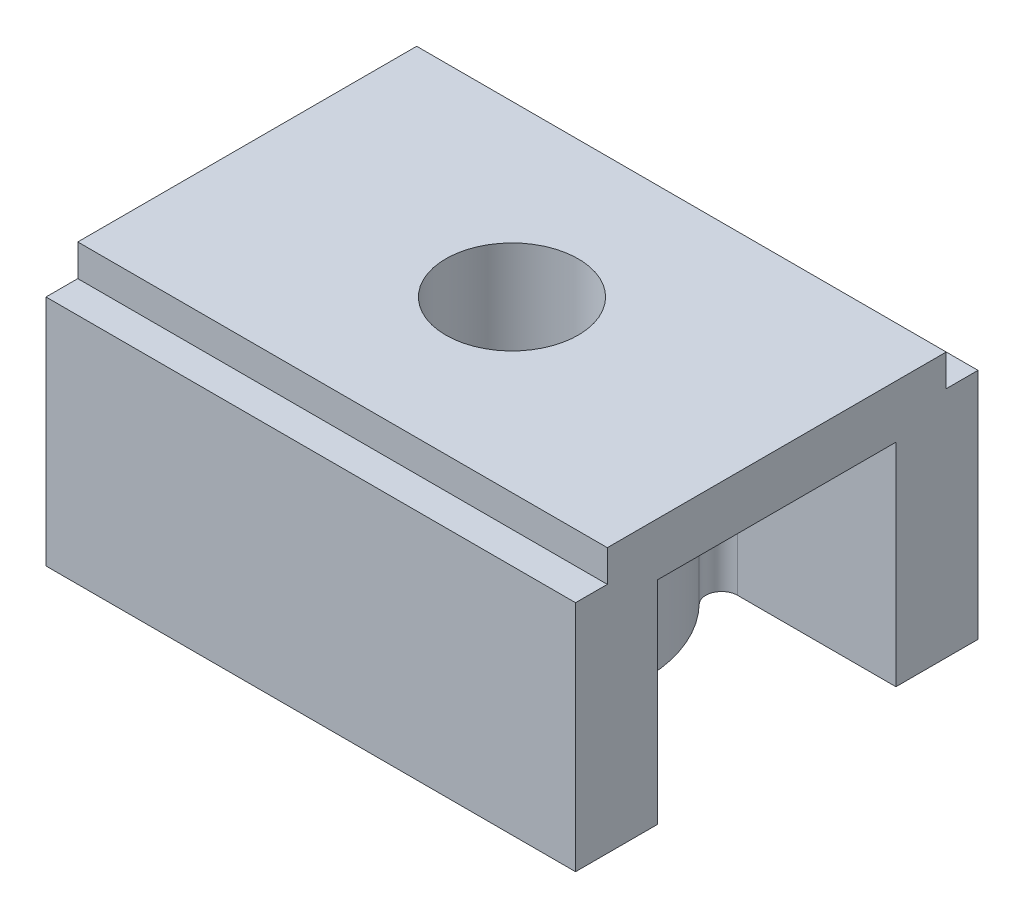
ISO-10303-21;
HEADER;
FILE_DESCRIPTION(('STEP AP214'),'2;1');
FILE_NAME('part.step','',(''),(''),'','','');
FILE_SCHEMA(('AUTOMOTIVE_DESIGN { 1 0 10303 214 1 1 1 1 }'));
ENDSEC;
DATA;
#1=APPLICATION_CONTEXT('core data for automotive mechanical design processes');
#2=APPLICATION_PROTOCOL_DEFINITION('international standard','automotive_design',2000,#1);
#3=PRODUCT_CONTEXT('',#1,'mechanical');
#4=PRODUCT('Part','Part','',(#3));
#5=PRODUCT_RELATED_PRODUCT_CATEGORY('part','',(#4));
#6=PRODUCT_DEFINITION_FORMATION('','',#4);
#7=PRODUCT_DEFINITION_CONTEXT('part definition',#1,'design');
#8=PRODUCT_DEFINITION('design','',#6,#7);
#9=PRODUCT_DEFINITION_SHAPE('','',#8);
#10=(LENGTH_UNIT() NAMED_UNIT(*) SI_UNIT(.MILLI.,.METRE.));
#11=(NAMED_UNIT(*) PLANE_ANGLE_UNIT() SI_UNIT($,.RADIAN.));
#12=(NAMED_UNIT(*) SI_UNIT($,.STERADIAN.) SOLID_ANGLE_UNIT());
#13=UNCERTAINTY_MEASURE_WITH_UNIT(LENGTH_MEASURE(1.E-05),#10,'distance_accuracy_value','');
#14=(GEOMETRIC_REPRESENTATION_CONTEXT(3) GLOBAL_UNCERTAINTY_ASSIGNED_CONTEXT((#13)) GLOBAL_UNIT_ASSIGNED_CONTEXT((#10,
#11,#12)) REPRESENTATION_CONTEXT('',''));
#15=CARTESIAN_POINT('',(0.,0.,0.));
#16=DIRECTION('',(0.,0.,1.));
#17=DIRECTION('',(1.,0.,0.));
#18=AXIS2_PLACEMENT_3D('',#15,#16,#17);
#19=CARTESIAN_POINT('',(-50.,40.,-38.));
#20=DIRECTION('',(0.,0.,-1.));
#21=DIRECTION('',(-1.,0.,0.));
#22=AXIS2_PLACEMENT_3D('',#19,#20,#21);
#23=PLANE('',#22);
#24=DIRECTION('',(0.,-1.,0.));
#25=VECTOR('',#24,1.);
#26=CARTESIAN_POINT('',(-50.,40.,-38.));
#27=LINE('',#26,#25);
#28=CARTESIAN_POINT('',(-50.,44.,-38.));
#29=VERTEX_POINT('',#28);
#30=CARTESIAN_POINT('',(-50.,0.,-38.));
#31=VERTEX_POINT('',#30);
#32=EDGE_CURVE('E195',#29,#31,#27,.T.);
#33=ORIENTED_EDGE('',*,*,#32,.F.);
#34=DIRECTION('',(-1.,0.,0.));
#35=VECTOR('',#34,1.);
#36=CARTESIAN_POINT('',(50.,44.,-38.));
#37=LINE('',#36,#35);
#38=CARTESIAN_POINT('',(50.,44.,-38.));
#39=VERTEX_POINT('',#38);
#40=EDGE_CURVE('E177',#39,#29,#37,.T.);
#41=ORIENTED_EDGE('',*,*,#40,.F.);
#42=DIRECTION('',(0.,-1.,0.));
#43=VECTOR('',#42,1.);
#44=CARTESIAN_POINT('',(50.,40.,-38.));
#45=LINE('',#44,#43);
#46=CARTESIAN_POINT('',(50.,0.,-38.));
#47=VERTEX_POINT('',#46);
#48=EDGE_CURVE('E188',#39,#47,#45,.T.);
#49=ORIENTED_EDGE('',*,*,#48,.T.);
#50=DIRECTION('',(1.,0.,0.));
#51=VECTOR('',#50,1.);
#52=CARTESIAN_POINT('',(-50.,0.,-38.));
#53=LINE('',#52,#51);
#54=EDGE_CURVE('E253',#31,#47,#53,.T.);
#55=ORIENTED_EDGE('',*,*,#54,.F.);
#56=EDGE_LOOP('',(#33,#41,#49,#55));
#57=FACE_BOUND('',#56,.T.);
#58=ADVANCED_FACE('F39',(#57),#23,.T.);
#59=CARTESIAN_POINT('',(-50.,40.,38.));
#60=DIRECTION('',(0.,0.,-1.));
#61=DIRECTION('',(-1.,0.,0.));
#62=AXIS2_PLACEMENT_3D('',#59,#60,#61);
#63=PLANE('',#62);
#64=DIRECTION('',(0.,-1.,0.));
#65=VECTOR('',#64,1.);
#66=CARTESIAN_POINT('',(50.,40.,38.));
#67=LINE('',#66,#65);
#68=CARTESIAN_POINT('',(50.,44.,38.));
#69=VERTEX_POINT('',#68);
#70=CARTESIAN_POINT('',(50.,0.,38.));
#71=VERTEX_POINT('',#70);
#72=EDGE_CURVE('E50',#69,#71,#67,.T.);
#73=ORIENTED_EDGE('',*,*,#72,.F.);
#74=DIRECTION('',(1.,0.,0.));
#75=VECTOR('',#74,1.);
#76=CARTESIAN_POINT('',(-50.,44.,38.));
#77=LINE('',#76,#75);
#78=CARTESIAN_POINT('',(-50.,44.,38.));
#79=VERTEX_POINT('',#78);
#80=EDGE_CURVE('E539',#79,#69,#77,.T.);
#81=ORIENTED_EDGE('',*,*,#80,.F.);
#82=DIRECTION('',(0.,-1.,0.));
#83=VECTOR('',#82,1.);
#84=CARTESIAN_POINT('',(-50.,40.,38.));
#85=LINE('',#84,#83);
#86=CARTESIAN_POINT('',(-50.,0.,38.));
#87=VERTEX_POINT('',#86);
#88=EDGE_CURVE('E11',#79,#87,#85,.T.);
#89=ORIENTED_EDGE('',*,*,#88,.T.);
#90=DIRECTION('',(1.,0.,0.));
#91=VECTOR('',#90,1.);
#92=CARTESIAN_POINT('',(-50.,0.,38.));
#93=LINE('',#92,#91);
#94=EDGE_CURVE('E226',#87,#71,#93,.T.);
#95=ORIENTED_EDGE('',*,*,#94,.T.);
#96=EDGE_LOOP('',(#73,#81,#89,#95));
#97=FACE_BOUND('',#96,.T.);
#98=ADVANCED_FACE('F41',(#97),#63,.F.);
#99=CARTESIAN_POINT('',(20.0935312974101,40.,22.5));
#100=DIRECTION('',(0.,0.,-1.));
#101=DIRECTION('',(-1.,0.,0.));
#102=AXIS2_PLACEMENT_3D('',#99,#100,#101);
#103=PLANE('',#102);
#104=DIRECTION('',(1.,0.,0.));
#105=VECTOR('',#104,1.);
#106=CARTESIAN_POINT('',(20.0935312974101,0.,22.5));
#107=LINE('',#106,#105);
#108=CARTESIAN_POINT('',(20.0935312974101,0.,22.5));
#109=VERTEX_POINT('',#108);
#110=CARTESIAN_POINT('',(50.,0.,22.5));
#111=VERTEX_POINT('',#110);
#112=EDGE_CURVE('E238',#109,#111,#107,.T.);
#113=ORIENTED_EDGE('',*,*,#112,.F.);
#114=DIRECTION('',(0.,-1.,0.));
#115=VECTOR('',#114,1.);
#116=CARTESIAN_POINT('',(20.0935312974101,40.,22.5));
#117=LINE('',#116,#115);
#118=CARTESIAN_POINT('',(20.0935312974101,40.,22.5));
#119=VERTEX_POINT('',#118);
#120=EDGE_CURVE('E215',#119,#109,#117,.T.);
#121=ORIENTED_EDGE('',*,*,#120,.F.);
#122=DIRECTION('',(1.,0.,0.));
#123=VECTOR('',#122,1.);
#124=CARTESIAN_POINT('',(20.0935312974101,40.,22.5));
#125=LINE('',#124,#123);
#126=CARTESIAN_POINT('',(50.,40.,22.5));
#127=VERTEX_POINT('',#126);
#128=EDGE_CURVE('E274',#119,#127,#125,.T.);
#129=ORIENTED_EDGE('',*,*,#128,.T.);
#130=DIRECTION('',(0.,-1.,0.));
#131=VECTOR('',#130,1.);
#132=CARTESIAN_POINT('',(50.,40.,22.5));
#133=LINE('',#132,#131);
#134=EDGE_CURVE('E211',#127,#111,#133,.T.);
#135=ORIENTED_EDGE('',*,*,#134,.T.);
#136=EDGE_LOOP('',(#113,#121,#129,#135));
#137=FACE_BOUND('',#136,.T.);
#138=ADVANCED_FACE('F361',(#137),#103,.T.);
#139=CARTESIAN_POINT('',(20.0935312974101,40.,19.5));
#140=DIRECTION('',(0.,-1.,0.));
#141=DIRECTION('',(0.,0.,-1.));
#142=AXIS2_PLACEMENT_3D('',#139,#140,#141);
#143=CYLINDRICAL_SURFACE('',#142,3.);
#144=CARTESIAN_POINT('',(20.0935312974101,0.,19.5));
#145=DIRECTION('',(0.,1.,0.));
#146=DIRECTION('',(0.,0.,1.));
#147=AXIS2_PLACEMENT_3D('',#144,#145,#146);
#148=CIRCLE('',#147,3.);
#149=CARTESIAN_POINT('',(17.9406529441162,0.,17.4107142857143));
#150=VERTEX_POINT('',#149);
#151=EDGE_CURVE('E239',#150,#109,#148,.T.);
#152=ORIENTED_EDGE('',*,*,#151,.F.);
#153=DIRECTION('',(0.,-1.,0.));
#154=VECTOR('',#153,1.);
#155=CARTESIAN_POINT('',(17.9406529441162,40.,17.4107142857143));
#156=LINE('',#155,#154);
#157=CARTESIAN_POINT('',(17.9406529441162,40.,17.4107142857143));
#158=VERTEX_POINT('',#157);
#159=EDGE_CURVE('E208',#158,#150,#156,.T.);
#160=ORIENTED_EDGE('',*,*,#159,.F.);
#161=CARTESIAN_POINT('',(20.0935312974101,40.,19.5));
#162=DIRECTION('',(0.,1.,0.));
#163=DIRECTION('',(0.,0.,1.));
#164=AXIS2_PLACEMENT_3D('',#161,#162,#163);
#165=CIRCLE('',#164,3.);
#166=EDGE_CURVE('E332',#158,#119,#165,.T.);
#167=ORIENTED_EDGE('',*,*,#166,.T.);
#168=ORIENTED_EDGE('',*,*,#120,.T.);
#169=EDGE_LOOP('',(#152,#160,#167,#168));
#170=FACE_BOUND('',#169,.T.);
#171=ADVANCED_FACE('F359',(#170),#143,.F.);
#172=CARTESIAN_POINT('',(0.,40.,0.));
#173=DIRECTION('',(0.,-1.,0.));
#174=DIRECTION('',(0.,0.,-1.));
#175=AXIS2_PLACEMENT_3D('',#172,#173,#174);
#176=CYLINDRICAL_SURFACE('',#175,25.);
#177=CARTESIAN_POINT('',(0.,0.,0.));
#178=DIRECTION('',(0.,1.,0.));
#179=DIRECTION('',(0.,0.,1.));
#180=AXIS2_PLACEMENT_3D('',#177,#178,#179);
#181=CIRCLE('',#180,25.);
#182=CARTESIAN_POINT('',(17.9406529441162,0.,-17.4107142857143));
#183=VERTEX_POINT('',#182);
#184=EDGE_CURVE('E244',#150,#183,#181,.T.);
#185=ORIENTED_EDGE('',*,*,#184,.T.);
#186=DIRECTION('',(0.,-1.,0.));
#187=VECTOR('',#186,1.);
#188=CARTESIAN_POINT('',(17.9406529441162,40.,-17.4107142857143));
#189=LINE('',#188,#187);
#190=CARTESIAN_POINT('',(17.9406529441162,40.,-17.4107142857143));
#191=VERTEX_POINT('',#190);
#192=EDGE_CURVE('E206',#191,#183,#189,.T.);
#193=ORIENTED_EDGE('',*,*,#192,.F.);
#194=CARTESIAN_POINT('',(0.,40.,0.));
#195=DIRECTION('',(0.,1.,0.));
#196=DIRECTION('',(0.,0.,1.));
#197=AXIS2_PLACEMENT_3D('',#194,#195,#196);
#198=CIRCLE('',#197,25.);
#199=EDGE_CURVE('E340',#158,#191,#198,.T.);
#200=ORIENTED_EDGE('',*,*,#199,.F.);
#201=ORIENTED_EDGE('',*,*,#159,.T.);
#202=EDGE_LOOP('',(#185,#193,#200,#201));
#203=FACE_BOUND('',#202,.T.);
#204=ADVANCED_FACE('F358',(#203),#176,.T.);
#205=CARTESIAN_POINT('',(20.0935312974101,40.,-19.5));
#206=DIRECTION('',(0.,-1.,0.));
#207=DIRECTION('',(0.,0.,-1.));
#208=AXIS2_PLACEMENT_3D('',#205,#206,#207);
#209=CYLINDRICAL_SURFACE('',#208,3.);
#210=CARTESIAN_POINT('',(20.0935312974101,0.,-19.5));
#211=DIRECTION('',(0.,1.,0.));
#212=DIRECTION('',(0.,0.,1.));
#213=AXIS2_PLACEMENT_3D('',#210,#211,#212);
#214=CIRCLE('',#213,3.);
#215=CARTESIAN_POINT('',(20.0935312974101,0.,-22.5));
#216=VERTEX_POINT('',#215);
#217=EDGE_CURVE('E247',#216,#183,#214,.T.);
#218=ORIENTED_EDGE('',*,*,#217,.F.);
#219=DIRECTION('',(0.,-1.,0.));
#220=VECTOR('',#219,1.);
#221=CARTESIAN_POINT('',(20.0935312974101,40.,-22.5));
#222=LINE('',#221,#220);
#223=CARTESIAN_POINT('',(20.0935312974101,40.,-22.5));
#224=VERTEX_POINT('',#223);
#225=EDGE_CURVE('E201',#224,#216,#222,.T.);
#226=ORIENTED_EDGE('',*,*,#225,.F.);
#227=CARTESIAN_POINT('',(20.0935312974101,40.,-19.5));
#228=DIRECTION('',(0.,1.,0.));
#229=DIRECTION('',(0.,0.,1.));
#230=AXIS2_PLACEMENT_3D('',#227,#228,#229);
#231=CIRCLE('',#230,3.);
#232=EDGE_CURVE('E339',#224,#191,#231,.T.);
#233=ORIENTED_EDGE('',*,*,#232,.T.);
#234=ORIENTED_EDGE('',*,*,#192,.T.);
#235=EDGE_LOOP('',(#218,#226,#233,#234));
#236=FACE_BOUND('',#235,.T.);
#237=ADVANCED_FACE('F355',(#236),#209,.F.);
#238=CARTESIAN_POINT('',(20.0935312974101,40.,-22.5));
#239=DIRECTION('',(0.,0.,-1.));
#240=DIRECTION('',(-1.,0.,0.));
#241=AXIS2_PLACEMENT_3D('',#238,#239,#240);
#242=PLANE('',#241);
#243=DIRECTION('',(1.,0.,0.));
#244=VECTOR('',#243,1.);
#245=CARTESIAN_POINT('',(20.0935312974101,0.,-22.5));
#246=LINE('',#245,#244);
#247=CARTESIAN_POINT('',(50.,0.,-22.5));
#248=VERTEX_POINT('',#247);
#249=EDGE_CURVE('E252',#216,#248,#246,.T.);
#250=ORIENTED_EDGE('',*,*,#249,.T.);
#251=DIRECTION('',(0.,-1.,0.));
#252=VECTOR('',#251,1.);
#253=CARTESIAN_POINT('',(50.,40.,-22.5));
#254=LINE('',#253,#252);
#255=CARTESIAN_POINT('',(50.,40.,-22.5));
#256=VERTEX_POINT('',#255);
#257=EDGE_CURVE('E196',#256,#248,#254,.T.);
#258=ORIENTED_EDGE('',*,*,#257,.F.);
#259=DIRECTION('',(1.,0.,0.));
#260=VECTOR('',#259,1.);
#261=CARTESIAN_POINT('',(20.0935312974101,40.,-22.5));
#262=LINE('',#261,#260);
#263=EDGE_CURVE('E307',#224,#256,#262,.T.);
#264=ORIENTED_EDGE('',*,*,#263,.F.);
#265=ORIENTED_EDGE('',*,*,#225,.T.);
#266=EDGE_LOOP('',(#250,#258,#264,#265));
#267=FACE_BOUND('',#266,.T.);
#268=ADVANCED_FACE('F350',(#267),#242,.F.);
#269=CARTESIAN_POINT('',(50.,40.,-38.));
#270=DIRECTION('',(1.,0.,0.));
#271=DIRECTION('',(0.,0.,-1.));
#272=AXIS2_PLACEMENT_3D('',#269,#270,#271);
#273=PLANE('',#272);
#274=DIRECTION('',(0.,1.,0.));
#275=VECTOR('',#274,1.);
#276=CARTESIAN_POINT('',(50.,44.,-32.));
#277=LINE('',#276,#275);
#278=CARTESIAN_POINT('',(50.,44.,-32.));
#279=VERTEX_POINT('',#278);
#280=CARTESIAN_POINT('',(50.,50.,-32.));
#281=VERTEX_POINT('',#280);
#282=EDGE_CURVE('E532',#279,#281,#277,.T.);
#283=ORIENTED_EDGE('',*,*,#282,.T.);
#284=DIRECTION('',(0.,0.,-1.));
#285=VECTOR('',#284,1.);
#286=CARTESIAN_POINT('',(50.,50.,-38.));
#287=LINE('',#286,#285);
#288=CARTESIAN_POINT('',(50.,50.,32.));
#289=VERTEX_POINT('',#288);
#290=EDGE_CURVE('E319',#289,#281,#287,.T.);
#291=ORIENTED_EDGE('',*,*,#290,.F.);
#292=DIRECTION('',(0.,1.,0.));
#293=VECTOR('',#292,1.);
#294=CARTESIAN_POINT('',(50.,44.,32.));
#295=LINE('',#294,#293);
#296=CARTESIAN_POINT('',(50.,44.,32.));
#297=VERTEX_POINT('',#296);
#298=EDGE_CURVE('E65',#297,#289,#295,.T.);
#299=ORIENTED_EDGE('',*,*,#298,.F.);
#300=DIRECTION('',(0.,0.,-1.));
#301=VECTOR('',#300,1.);
#302=CARTESIAN_POINT('',(50.,44.,38.));
#303=LINE('',#302,#301);
#304=EDGE_CURVE('E222',#69,#297,#303,.T.);
#305=ORIENTED_EDGE('',*,*,#304,.F.);
#306=ORIENTED_EDGE('',*,*,#72,.T.);
#307=DIRECTION('',(0.,0.,1.));
#308=VECTOR('',#307,1.);
#309=CARTESIAN_POINT('',(50.,0.,22.5));
#310=LINE('',#309,#308);
#311=EDGE_CURVE('E221',#111,#71,#310,.T.);
#312=ORIENTED_EDGE('',*,*,#311,.F.);
#313=ORIENTED_EDGE('',*,*,#134,.F.);
#314=DIRECTION('',(0.,0.,-1.));
#315=VECTOR('',#314,1.);
#316=CARTESIAN_POINT('',(50.,40.,-38.));
#317=LINE('',#316,#315);
#318=EDGE_CURVE('E330',#127,#256,#317,.T.);
#319=ORIENTED_EDGE('',*,*,#318,.T.);
#320=ORIENTED_EDGE('',*,*,#257,.T.);
#321=DIRECTION('',(0.,0.,1.));
#322=VECTOR('',#321,1.);
#323=CARTESIAN_POINT('',(50.,0.,-38.));
#324=LINE('',#323,#322);
#325=EDGE_CURVE('E200',#47,#248,#324,.T.);
#326=ORIENTED_EDGE('',*,*,#325,.F.);
#327=ORIENTED_EDGE('',*,*,#48,.F.);
#328=DIRECTION('',(0.,0.,-1.));
#329=VECTOR('',#328,1.);
#330=CARTESIAN_POINT('',(50.,44.,-32.));
#331=LINE('',#330,#329);
#332=EDGE_CURVE('E176',#279,#39,#331,.T.);
#333=ORIENTED_EDGE('',*,*,#332,.F.);
#334=EDGE_LOOP('',(#283,#291,#299,#305,#306,#312,#313,#319,#320,#326,#327,#333));
#335=FACE_BOUND('',#334,.T.);
#336=ADVANCED_FACE('F193',(#335),#273,.T.);
#337=CARTESIAN_POINT('',(-50.,40.,-38.));
#338=DIRECTION('',(1.,0.,0.));
#339=DIRECTION('',(0.,0.,-1.));
#340=AXIS2_PLACEMENT_3D('',#337,#338,#339);
#341=PLANE('',#340);
#342=DIRECTION('',(0.,0.,1.));
#343=VECTOR('',#342,1.);
#344=CARTESIAN_POINT('',(-50.,50.,-38.));
#345=LINE('',#344,#343);
#346=CARTESIAN_POINT('',(-50.,50.,-32.));
#347=VERTEX_POINT('',#346);
#348=CARTESIAN_POINT('',(-50.,50.,32.));
#349=VERTEX_POINT('',#348);
#350=EDGE_CURVE('E317',#347,#349,#345,.T.);
#351=ORIENTED_EDGE('',*,*,#350,.F.);
#352=DIRECTION('',(0.,1.,0.));
#353=VECTOR('',#352,1.);
#354=CARTESIAN_POINT('',(-50.,44.,-32.));
#355=LINE('',#354,#353);
#356=CARTESIAN_POINT('',(-50.,44.,-32.));
#357=VERTEX_POINT('',#356);
#358=EDGE_CURVE('E53',#357,#347,#355,.T.);
#359=ORIENTED_EDGE('',*,*,#358,.F.);
#360=DIRECTION('',(0.,0.,1.));
#361=VECTOR('',#360,1.);
#362=CARTESIAN_POINT('',(-50.,44.,-38.));
#363=LINE('',#362,#361);
#364=EDGE_CURVE('E194',#29,#357,#363,.T.);
#365=ORIENTED_EDGE('',*,*,#364,.F.);
#366=ORIENTED_EDGE('',*,*,#32,.T.);
#367=DIRECTION('',(0.,0.,1.));
#368=VECTOR('',#367,1.);
#369=CARTESIAN_POINT('',(-50.,0.,-38.));
#370=LINE('',#369,#368);
#371=CARTESIAN_POINT('',(-50.,0.,-22.5));
#372=VERTEX_POINT('',#371);
#373=EDGE_CURVE('E260',#31,#372,#370,.T.);
#374=ORIENTED_EDGE('',*,*,#373,.T.);
#375=DIRECTION('',(0.,-1.,0.));
#376=VECTOR('',#375,1.);
#377=CARTESIAN_POINT('',(-50.,40.,-22.5));
#378=LINE('',#377,#376);
#379=CARTESIAN_POINT('',(-50.,40.,-22.5));
#380=VERTEX_POINT('',#379);
#381=EDGE_CURVE('E203',#380,#372,#378,.T.);
#382=ORIENTED_EDGE('',*,*,#381,.F.);
#383=DIRECTION('',(0.,0.,1.));
#384=VECTOR('',#383,1.);
#385=CARTESIAN_POINT('',(-50.,40.,-38.));
#386=LINE('',#385,#384);
#387=CARTESIAN_POINT('',(-50.,40.,22.5));
#388=VERTEX_POINT('',#387);
#389=EDGE_CURVE('E324',#380,#388,#386,.T.);
#390=ORIENTED_EDGE('',*,*,#389,.T.);
#391=DIRECTION('',(0.,-1.,0.));
#392=VECTOR('',#391,1.);
#393=CARTESIAN_POINT('',(-50.,40.,22.5));
#394=LINE('',#393,#392);
#395=CARTESIAN_POINT('',(-50.,0.,22.5));
#396=VERTEX_POINT('',#395);
#397=EDGE_CURVE('E273',#388,#396,#394,.T.);
#398=ORIENTED_EDGE('',*,*,#397,.T.);
#399=DIRECTION('',(0.,0.,1.));
#400=VECTOR('',#399,1.);
#401=CARTESIAN_POINT('',(-50.,0.,22.5));
#402=LINE('',#401,#400);
#403=EDGE_CURVE('E231',#396,#87,#402,.T.);
#404=ORIENTED_EDGE('',*,*,#403,.T.);
#405=ORIENTED_EDGE('',*,*,#88,.F.);
#406=DIRECTION('',(0.,0.,1.));
#407=VECTOR('',#406,1.);
#408=CARTESIAN_POINT('',(-50.,44.,32.));
#409=LINE('',#408,#407);
#410=CARTESIAN_POINT('',(-50.,44.,32.));
#411=VERTEX_POINT('',#410);
#412=EDGE_CURVE('E541',#411,#79,#409,.T.);
#413=ORIENTED_EDGE('',*,*,#412,.F.);
#414=DIRECTION('',(0.,1.,0.));
#415=VECTOR('',#414,1.);
#416=CARTESIAN_POINT('',(-50.,44.,32.));
#417=LINE('',#416,#415);
#418=EDGE_CURVE('E540',#411,#349,#417,.T.);
#419=ORIENTED_EDGE('',*,*,#418,.T.);
#420=EDGE_LOOP('',(#351,#359,#365,#366,#374,#382,#390,#398,#404,#405,#413,#419));
#421=FACE_BOUND('',#420,.T.);
#422=ADVANCED_FACE('F380',(#421),#341,.F.);
#423=CARTESIAN_POINT('',(-50.,40.,-22.5));
#424=DIRECTION('',(0.,0.,-1.));
#425=DIRECTION('',(-1.,0.,0.));
#426=AXIS2_PLACEMENT_3D('',#423,#424,#425);
#427=PLANE('',#426);
#428=DIRECTION('',(1.,0.,0.));
#429=VECTOR('',#428,1.);
#430=CARTESIAN_POINT('',(-50.,0.,-22.5));
#431=LINE('',#430,#429);
#432=CARTESIAN_POINT('',(-20.0935312974102,0.,-22.5));
#433=VERTEX_POINT('',#432);
#434=EDGE_CURVE('E256',#372,#433,#431,.T.);
#435=ORIENTED_EDGE('',*,*,#434,.T.);
#436=DIRECTION('',(0.,-1.,0.));
#437=VECTOR('',#436,1.);
#438=CARTESIAN_POINT('',(-20.0935312974102,40.,-22.5));
#439=LINE('',#438,#437);
#440=CARTESIAN_POINT('',(-20.0935312974102,40.,-22.5));
#441=VERTEX_POINT('',#440);
#442=EDGE_CURVE('E281',#441,#433,#439,.T.);
#443=ORIENTED_EDGE('',*,*,#442,.F.);
#444=DIRECTION('',(1.,0.,0.));
#445=VECTOR('',#444,1.);
#446=CARTESIAN_POINT('',(-50.,40.,-22.5));
#447=LINE('',#446,#445);
#448=EDGE_CURVE('E292',#380,#441,#447,.T.);
#449=ORIENTED_EDGE('',*,*,#448,.F.);
#450=ORIENTED_EDGE('',*,*,#381,.T.);
#451=EDGE_LOOP('',(#435,#443,#449,#450));
#452=FACE_BOUND('',#451,.T.);
#453=ADVANCED_FACE('F289',(#452),#427,.F.);
#454=CARTESIAN_POINT('',(-20.0935312974102,40.,-19.5));
#455=DIRECTION('',(0.,-1.,0.));
#456=DIRECTION('',(0.,0.,-1.));
#457=AXIS2_PLACEMENT_3D('',#454,#455,#456);
#458=CYLINDRICAL_SURFACE('',#457,3.00000000000001);
#459=CARTESIAN_POINT('',(-20.0935312974102,0.,-19.5));
#460=DIRECTION('',(0.,1.,0.));
#461=DIRECTION('',(0.,0.,1.));
#462=AXIS2_PLACEMENT_3D('',#459,#460,#461);
#463=CIRCLE('',#462,3.00000000000001);
#464=CARTESIAN_POINT('',(-17.9406529441162,0.,-17.4107142857143));
#465=VERTEX_POINT('',#464);
#466=EDGE_CURVE('E265',#465,#433,#463,.T.);
#467=ORIENTED_EDGE('',*,*,#466,.F.);
#468=DIRECTION('',(0.,-1.,0.));
#469=VECTOR('',#468,1.);
#470=CARTESIAN_POINT('',(-17.9406529441162,40.,-17.4107142857143));
#471=LINE('',#470,#469);
#472=CARTESIAN_POINT('',(-17.9406529441162,40.,-17.4107142857143));
#473=VERTEX_POINT('',#472);
#474=EDGE_CURVE('E285',#473,#465,#471,.T.);
#475=ORIENTED_EDGE('',*,*,#474,.F.);
#476=CARTESIAN_POINT('',(-20.0935312974102,40.,-19.5));
#477=DIRECTION('',(0.,1.,0.));
#478=DIRECTION('',(0.,0.,1.));
#479=AXIS2_PLACEMENT_3D('',#476,#477,#478);
#480=CIRCLE('',#479,3.00000000000001);
#481=EDGE_CURVE('E303',#473,#441,#480,.T.);
#482=ORIENTED_EDGE('',*,*,#481,.T.);
#483=ORIENTED_EDGE('',*,*,#442,.T.);
#484=EDGE_LOOP('',(#467,#475,#482,#483));
#485=FACE_BOUND('',#484,.T.);
#486=ADVANCED_FACE('F297',(#485),#458,.F.);
#487=CARTESIAN_POINT('',(0.,40.,0.));
#488=DIRECTION('',(0.,-1.,0.));
#489=DIRECTION('',(0.,0.,-1.));
#490=AXIS2_PLACEMENT_3D('',#487,#488,#489);
#491=CYLINDRICAL_SURFACE('',#490,25.);
#492=CARTESIAN_POINT('',(0.,0.,0.));
#493=DIRECTION('',(0.,1.,0.));
#494=DIRECTION('',(0.,0.,1.));
#495=AXIS2_PLACEMENT_3D('',#492,#493,#494);
#496=CIRCLE('',#495,25.);
#497=CARTESIAN_POINT('',(-17.9406529441162,0.,17.4107142857143));
#498=VERTEX_POINT('',#497);
#499=EDGE_CURVE('E263',#465,#498,#496,.T.);
#500=ORIENTED_EDGE('',*,*,#499,.T.);
#501=DIRECTION('',(0.,-1.,0.));
#502=VECTOR('',#501,1.);
#503=CARTESIAN_POINT('',(-17.9406529441162,40.,17.4107142857143));
#504=LINE('',#503,#502);
#505=CARTESIAN_POINT('',(-17.9406529441162,40.,17.4107142857143));
#506=VERTEX_POINT('',#505);
#507=EDGE_CURVE('E278',#506,#498,#504,.T.);
#508=ORIENTED_EDGE('',*,*,#507,.F.);
#509=CARTESIAN_POINT('',(0.,40.,0.));
#510=DIRECTION('',(0.,1.,0.));
#511=DIRECTION('',(0.,0.,1.));
#512=AXIS2_PLACEMENT_3D('',#509,#510,#511);
#513=CIRCLE('',#512,25.);
#514=EDGE_CURVE('E304',#473,#506,#513,.T.);
#515=ORIENTED_EDGE('',*,*,#514,.F.);
#516=ORIENTED_EDGE('',*,*,#474,.T.);
#517=EDGE_LOOP('',(#500,#508,#515,#516));
#518=FACE_BOUND('',#517,.T.);
#519=ADVANCED_FACE('F413',(#518),#491,.T.);
#520=CARTESIAN_POINT('',(-20.0935312974101,40.,19.5));
#521=DIRECTION('',(0.,-1.,0.));
#522=DIRECTION('',(0.,0.,-1.));
#523=AXIS2_PLACEMENT_3D('',#520,#521,#522);
#524=CYLINDRICAL_SURFACE('',#523,3.);
#525=CARTESIAN_POINT('',(-20.0935312974101,0.,19.5));
#526=DIRECTION('',(0.,1.,0.));
#527=DIRECTION('',(0.,0.,1.));
#528=AXIS2_PLACEMENT_3D('',#525,#526,#527);
#529=CIRCLE('',#528,3.);
#530=CARTESIAN_POINT('',(-20.0935312974101,0.,22.5));
#531=VERTEX_POINT('',#530);
#532=EDGE_CURVE('E268',#531,#498,#529,.T.);
#533=ORIENTED_EDGE('',*,*,#532,.F.);
#534=DIRECTION('',(0.,-1.,0.));
#535=VECTOR('',#534,1.);
#536=CARTESIAN_POINT('',(-20.0935312974101,40.,22.5));
#537=LINE('',#536,#535);
#538=CARTESIAN_POINT('',(-20.0935312974101,40.,22.5));
#539=VERTEX_POINT('',#538);
#540=EDGE_CURVE('E280',#539,#531,#537,.T.);
#541=ORIENTED_EDGE('',*,*,#540,.F.);
#542=CARTESIAN_POINT('',(-20.0935312974101,40.,19.5));
#543=DIRECTION('',(0.,1.,0.));
#544=DIRECTION('',(0.,0.,1.));
#545=AXIS2_PLACEMENT_3D('',#542,#543,#544);
#546=CIRCLE('',#545,3.);
#547=EDGE_CURVE('E310',#539,#506,#546,.T.);
#548=ORIENTED_EDGE('',*,*,#547,.T.);
#549=ORIENTED_EDGE('',*,*,#507,.T.);
#550=EDGE_LOOP('',(#533,#541,#548,#549));
#551=FACE_BOUND('',#550,.T.);
#552=ADVANCED_FACE('F421',(#551),#524,.F.);
#553=CARTESIAN_POINT('',(-50.,40.,22.5));
#554=DIRECTION('',(0.,0.,-1.));
#555=DIRECTION('',(-1.,0.,0.));
#556=AXIS2_PLACEMENT_3D('',#553,#554,#555);
#557=PLANE('',#556);
#558=DIRECTION('',(1.,0.,0.));
#559=VECTOR('',#558,1.);
#560=CARTESIAN_POINT('',(-50.,0.,22.5));
#561=LINE('',#560,#559);
#562=EDGE_CURVE('E272',#396,#531,#561,.T.);
#563=ORIENTED_EDGE('',*,*,#562,.F.);
#564=ORIENTED_EDGE('',*,*,#397,.F.);
#565=DIRECTION('',(1.,0.,0.));
#566=VECTOR('',#565,1.);
#567=CARTESIAN_POINT('',(-50.,40.,22.5));
#568=LINE('',#567,#566);
#569=EDGE_CURVE('E279',#388,#539,#568,.T.);
#570=ORIENTED_EDGE('',*,*,#569,.T.);
#571=ORIENTED_EDGE('',*,*,#540,.T.);
#572=EDGE_LOOP('',(#563,#564,#570,#571));
#573=FACE_BOUND('',#572,.T.);
#574=ADVANCED_FACE('F435',(#573),#557,.T.);
#575=CARTESIAN_POINT('',(20.0935312974101,0.,19.5));
#576=DIRECTION('',(0.,1.,0.));
#577=DIRECTION('',(0.,0.,1.));
#578=AXIS2_PLACEMENT_3D('',#575,#576,#577);
#579=PLANE('',#578);
#580=CARTESIAN_POINT('',(0.,0.,0.));
#581=DIRECTION('',(0.,1.,0.));
#582=DIRECTION('',(0.,0.,1.));
#583=AXIS2_PLACEMENT_3D('',#580,#581,#582);
#584=CIRCLE('',#583,12.5);
#585=CARTESIAN_POINT('',(0.,0.,12.5));
#586=VERTEX_POINT('',#585);
#587=EDGE_CURVE('E328',#586,#586,#584,.T.);
#588=ORIENTED_EDGE('',*,*,#587,.T.);
#589=EDGE_LOOP('',(#588));
#590=FACE_BOUND('',#589,.T.);
#591=ORIENTED_EDGE('',*,*,#403,.F.);
#592=ORIENTED_EDGE('',*,*,#562,.T.);
#593=ORIENTED_EDGE('',*,*,#532,.T.);
#594=ORIENTED_EDGE('',*,*,#499,.F.);
#595=ORIENTED_EDGE('',*,*,#466,.T.);
#596=ORIENTED_EDGE('',*,*,#434,.F.);
#597=ORIENTED_EDGE('',*,*,#373,.F.);
#598=ORIENTED_EDGE('',*,*,#54,.T.);
#599=ORIENTED_EDGE('',*,*,#325,.T.);
#600=ORIENTED_EDGE('',*,*,#249,.F.);
#601=ORIENTED_EDGE('',*,*,#217,.T.);
#602=ORIENTED_EDGE('',*,*,#184,.F.);
#603=ORIENTED_EDGE('',*,*,#151,.T.);
#604=ORIENTED_EDGE('',*,*,#112,.T.);
#605=ORIENTED_EDGE('',*,*,#311,.T.);
#606=ORIENTED_EDGE('',*,*,#94,.F.);
#607=EDGE_LOOP('',(#591,#592,#593,#594,#595,#596,#597,#598,#599,#600,#601,#602,#603,#604,#605,#606));
#608=FACE_BOUND('',#607,.T.);
#609=ADVANCED_FACE('F232',(#590,#608),#579,.F.);
#610=CARTESIAN_POINT('',(0.,40.,0.));
#611=DIRECTION('',(0.,1.,0.));
#612=DIRECTION('',(0.,0.,1.));
#613=AXIS2_PLACEMENT_3D('',#610,#611,#612);
#614=PLANE('',#613);
#615=ORIENTED_EDGE('',*,*,#389,.F.);
#616=ORIENTED_EDGE('',*,*,#448,.T.);
#617=ORIENTED_EDGE('',*,*,#481,.F.);
#618=ORIENTED_EDGE('',*,*,#514,.T.);
#619=ORIENTED_EDGE('',*,*,#547,.F.);
#620=ORIENTED_EDGE('',*,*,#569,.F.);
#621=EDGE_LOOP('',(#615,#616,#617,#618,#619,#620));
#622=FACE_BOUND('',#621,.T.);
#623=ADVANCED_FACE('F450',(#622),#614,.F.);
#624=CARTESIAN_POINT('',(0.,50.,0.));
#625=DIRECTION('',(0.,1.,0.));
#626=DIRECTION('',(0.,0.,1.));
#627=AXIS2_PLACEMENT_3D('',#624,#625,#626);
#628=PLANE('',#627);
#629=DIRECTION('',(1.,0.,0.));
#630=VECTOR('',#629,1.);
#631=CARTESIAN_POINT('',(-50.,50.,-32.));
#632=LINE('',#631,#630);
#633=EDGE_CURVE('E184',#347,#281,#632,.T.);
#634=ORIENTED_EDGE('',*,*,#633,.F.);
#635=ORIENTED_EDGE('',*,*,#350,.T.);
#636=DIRECTION('',(-1.,0.,0.));
#637=VECTOR('',#636,1.);
#638=CARTESIAN_POINT('',(-50.,50.,32.));
#639=LINE('',#638,#637);
#640=EDGE_CURVE('E542',#289,#349,#639,.T.);
#641=ORIENTED_EDGE('',*,*,#640,.F.);
#642=ORIENTED_EDGE('',*,*,#290,.T.);
#643=EDGE_LOOP('',(#634,#635,#641,#642));
#644=FACE_BOUND('',#643,.T.);
#645=CARTESIAN_POINT('',(0.,50.,0.));
#646=DIRECTION('',(0.,1.,0.));
#647=DIRECTION('',(0.,0.,1.));
#648=AXIS2_PLACEMENT_3D('',#645,#646,#647);
#649=CIRCLE('',#648,12.5);
#650=CARTESIAN_POINT('',(0.,50.,12.5));
#651=VERTEX_POINT('',#650);
#652=EDGE_CURVE('E529',#651,#651,#649,.T.);
#653=ORIENTED_EDGE('',*,*,#652,.F.);
#654=EDGE_LOOP('',(#653));
#655=FACE_BOUND('',#654,.T.);
#656=ADVANCED_FACE('F452',(#644,#655),#628,.T.);
#657=ORIENTED_EDGE('',*,*,#128,.F.);
#658=ORIENTED_EDGE('',*,*,#166,.F.);
#659=ORIENTED_EDGE('',*,*,#199,.T.);
#660=ORIENTED_EDGE('',*,*,#232,.F.);
#661=ORIENTED_EDGE('',*,*,#263,.T.);
#662=ORIENTED_EDGE('',*,*,#318,.F.);
#663=EDGE_LOOP('',(#657,#658,#659,#660,#661,#662));
#664=FACE_BOUND('',#663,.T.);
#665=ADVANCED_FACE('F344',(#664),#614,.F.);
#666=CARTESIAN_POINT('',(0.,-6.00000000000001,0.));
#667=DIRECTION('',(0.,1.,0.));
#668=DIRECTION('',(0.,0.,1.));
#669=AXIS2_PLACEMENT_3D('',#666,#667,#668);
#670=CYLINDRICAL_SURFACE('',#669,12.5);
#671=ORIENTED_EDGE('',*,*,#652,.T.);
#672=EDGE_LOOP('',(#671));
#673=FACE_BOUND('',#672,.T.);
#674=ORIENTED_EDGE('',*,*,#587,.F.);
#675=EDGE_LOOP('',(#674));
#676=FACE_BOUND('',#675,.T.);
#677=ADVANCED_FACE('F461',(#673,#676),#670,.F.);
#678=CARTESIAN_POINT('',(-50.,44.,32.));
#679=DIRECTION('',(0.,0.,-1.));
#680=DIRECTION('',(-1.,0.,0.));
#681=AXIS2_PLACEMENT_3D('',#678,#679,#680);
#682=PLANE('',#681);
#683=ORIENTED_EDGE('',*,*,#640,.T.);
#684=ORIENTED_EDGE('',*,*,#418,.F.);
#685=DIRECTION('',(-1.,0.,0.));
#686=VECTOR('',#685,1.);
#687=CARTESIAN_POINT('',(-50.,44.,32.));
#688=LINE('',#687,#686);
#689=EDGE_CURVE('E546',#297,#411,#688,.T.);
#690=ORIENTED_EDGE('',*,*,#689,.F.);
#691=ORIENTED_EDGE('',*,*,#298,.T.);
#692=EDGE_LOOP('',(#683,#684,#690,#691));
#693=FACE_BOUND('',#692,.T.);
#694=ADVANCED_FACE('F471',(#693),#682,.F.);
#695=CARTESIAN_POINT('',(0.,44.,0.));
#696=DIRECTION('',(0.,-1.,0.));
#697=DIRECTION('',(0.,0.,-1.));
#698=AXIS2_PLACEMENT_3D('',#695,#696,#697);
#699=PLANE('',#698);
#700=ORIENTED_EDGE('',*,*,#304,.T.);
#701=ORIENTED_EDGE('',*,*,#689,.T.);
#702=ORIENTED_EDGE('',*,*,#412,.T.);
#703=ORIENTED_EDGE('',*,*,#80,.T.);
#704=EDGE_LOOP('',(#700,#701,#702,#703));
#705=FACE_BOUND('',#704,.T.);
#706=ADVANCED_FACE('F494',(#705),#699,.F.);
#707=CARTESIAN_POINT('',(-50.,44.,-32.));
#708=DIRECTION('',(0.,0.,1.));
#709=DIRECTION('',(1.,0.,0.));
#710=AXIS2_PLACEMENT_3D('',#707,#708,#709);
#711=PLANE('',#710);
#712=ORIENTED_EDGE('',*,*,#633,.T.);
#713=ORIENTED_EDGE('',*,*,#282,.F.);
#714=DIRECTION('',(1.,0.,0.));
#715=VECTOR('',#714,1.);
#716=CARTESIAN_POINT('',(-50.,44.,-32.));
#717=LINE('',#716,#715);
#718=EDGE_CURVE('E181',#357,#279,#717,.T.);
#719=ORIENTED_EDGE('',*,*,#718,.F.);
#720=ORIENTED_EDGE('',*,*,#358,.T.);
#721=EDGE_LOOP('',(#712,#713,#719,#720));
#722=FACE_BOUND('',#721,.T.);
#723=ADVANCED_FACE('F502',(#722),#711,.F.);
#724=CARTESIAN_POINT('',(0.,44.,0.));
#725=DIRECTION('',(0.,1.,0.));
#726=DIRECTION('',(0.,0.,1.));
#727=AXIS2_PLACEMENT_3D('',#724,#725,#726);
#728=PLANE('',#727);
#729=ORIENTED_EDGE('',*,*,#332,.T.);
#730=ORIENTED_EDGE('',*,*,#40,.T.);
#731=ORIENTED_EDGE('',*,*,#364,.T.);
#732=ORIENTED_EDGE('',*,*,#718,.T.);
#733=EDGE_LOOP('',(#729,#730,#731,#732));
#734=FACE_BOUND('',#733,.T.);
#735=ADVANCED_FACE('F178',(#734),#728,.T.);
#736=CLOSED_SHELL('',(#58,#98,#138,#171,#204,#237,#268,#336,#422,#453,#486,#519,#552,#574,#609,
#623,#656,#665,#677,#694,#706,#723,#735));
#737=MANIFOLD_SOLID_BREP('B2',#736);
#738=ADVANCED_BREP_SHAPE_REPRESENTATION('',(#18,#737),#14);
#739=SHAPE_DEFINITION_REPRESENTATION(#9,#738);
ENDSEC;
END-ISO-10303-21;
